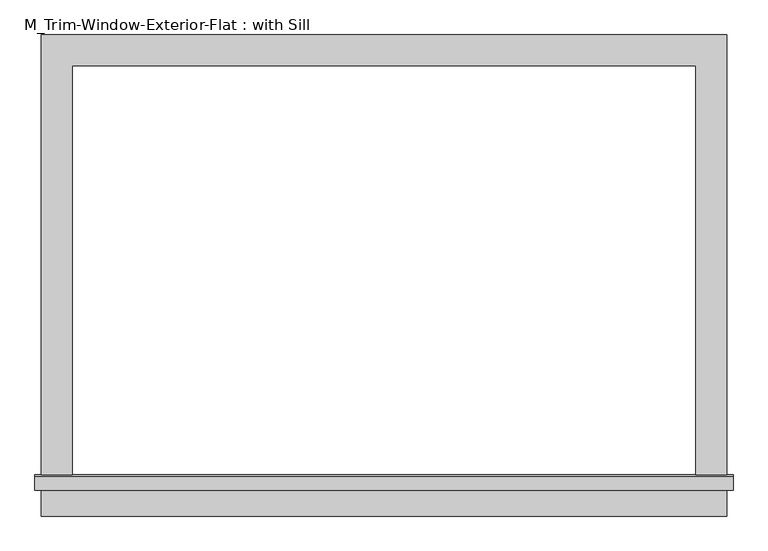
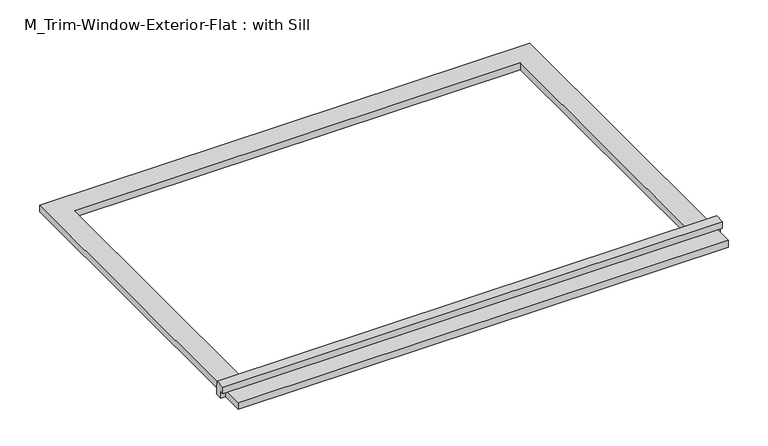
"""IFC4 building model written with IfcOpenShell, lengths in millimetres: proxy geometry, M_Trim-Window-Exterior-Flat : with Sill."""

from ifc_helpers import new_model, si_unit, frame, origin, origin_with_axes, place, context, project, spatial, polyline, outline, extrude, source, transform, mapped, element, save


def m_trim_window_exterior_flat_with_sill_3a557199(model_context):
    return source(origin(), model_context, "Body", "SweptSolid", [
        extrude(outline(polyline([(669.6, -820.4323709), (669.6, -880.4323709), (-669.6, -880.4323709), (-669.6, -820.4323709), (669.6, -820.4323709)])), origin_with_axes(), (0.0, 0.0, 1.0), 19.05),
        extrude(outline(polyline([(-830.0, 38.1), (-802.4580645, 38.1), (-800.0, 19.05), (-800.0, 0.0), (-820.4323709, 0.0), (-820.4323709, 19.05), (-830.0, 19.05), (-830.0, 38.1)])), frame((-682.3, 0.0, 0.0), z_axis=(1.0, 0.0, 0.0), x_axis=(0.0, 1.0, 0.0)), (0.0, 0.0, 1.0), 1364.6),
        extrude(outline(polyline([(-669.6, 60.0), (669.6, 60.0), (669.6, -800.0), (609.6, -800.0), (609.6, 0.0), (-609.6, 0.0), (-609.6, -800.0), (-669.6, -800.0), (-669.6, 60.0)])), origin_with_axes(), (0.0, 0.0, 1.0), 19.05),
    ])


if __name__ == "__main__":
    model = new_model("IFC4")
    model_context = context("Model", 3, world=origin())
    ifc_project = project(units=[si_unit("LENGTHUNIT", "METRE", prefix="MILLI")], contexts=[model_context])
    site = spatial("IfcSite", under=ifc_project)
    building = spatial("IfcBuilding", under=site)
    placement = place(None, origin())
    m_trim_window_exterior_flat_with_sill_shape = m_trim_window_exterior_flat_with_sill_3a557199(model_context)
    element("IfcBuildingElementProxy", 1, Name="M_Trim-Window-Exterior-Flat : with Sill", ObjectType="M_Trim-Window-Exterior-Flat : with Sill", at=placement, inside=building, context=model_context, shape_type="MappedRepresentation", body=[
        mapped(m_trim_window_exterior_flat_with_sill_shape, transform((0.0, 0.0, 0.0), x_axis=(1.0, 0.0, 0.0), y_axis=(0.0, 1.0, 0.0), z_axis=(0.0, 0.0, 1.0))),
    ])
    save(model, "model.ifc")

# Revit data of these elements
# Type "M_Trim-Window-Exterior-Flat : with Sill"
#   Trim Width = 0' - 2.3622"
#   Trim Thickness_Picture Frame = 0' - 1.1811"
#   Trim Thickness_with Sill = 0' - 0 3/4"
#   Sill Thickness = 0' - 1.1811"
#   Opening Width [instance default] = 1' - 11.62205"
#   Opening Height [instance default] = 2' - 11.43307"
#   Default Elevation = 3' - 11.24409"
#   Sill = yes
#   Picture Frame = no
#   Trim Material [instance default] = none
# Element 1 (IfcBuildingElementProxy, "M_Trim-Window-Exterior-Flat : with Sill")
#   Opening Width = 4' - 0"
#   Opening Height = 2' - 7.49606"
#   Trim Material = Clad - White
#   Materials on its faces: "Clad - White"
# Materials
#   "Clad - White": class "Wood", colour RGB 242 242 238, transparency 0, Cost = 0
